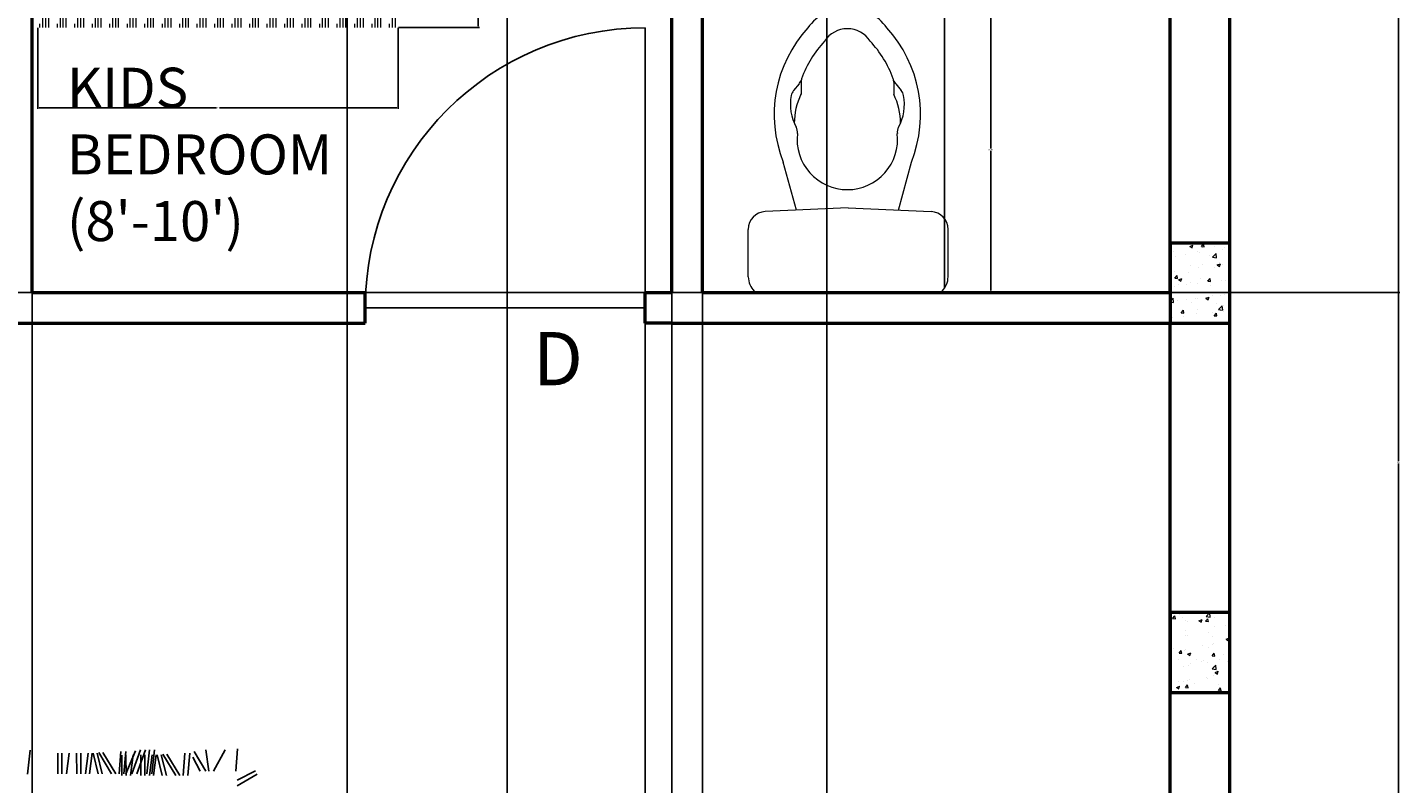
# Model space of a CAD drawing. Units: inches. Extents: x -1517 to -668, y -425 to 52.
# Tile 7 of 13: x -1186 to -980, y -176 to -63. Entities that reach past the tile are written whole.
import ezdxf

# ---------------------------------------------------------------- set-up
doc = ezdxf.new("R2010")
doc.units = ezdxf.units.IN
doc.header["$MEASUREMENT"] = 0
for name, color, linetype, lineweight in [('A-ANNO-DIMS', 2, 'Continuous', 18), ('A-ANNO-TEXT', 7, 'Continuous', 18), ('A-AREA-IDEN', 7, 'Continuous', 25), ('A-COLS-PATT', 252, 'Continuous', 13), ('A-FLOR-FIXT', 9, 'Continuous', 18), ('column', 7, 'Continuous', 50), ('doors', 25, 'Continuous', 25), ('furniture block', 8, 'Continuous', 18), ('walls', 240, 'Continuous', 50)]:
    doc.layers.add(name, color=color, linetype=linetype, lineweight=lineweight)
doc.layers.add('辅助线', color=1, linetype='Continuous')
doc.styles.get("Standard").update_dxf_attribs({"font": 'arial.ttf'})
doc.dimstyles.get("Standard").update_dxf_attribs({"dimtxt": 0.18, "dimasz": 0.18, "dimexe": 0.18, "dimexo": 0.0625, "dimgap": 0.09, "dimtad": 0, "dimtih": 1, "dimtoh": 1, "dimdec": 4, "dimzin": 0, "dimdsep": 46, "dimlunit": 4, "dimtxsty": 'Standard', "dimcen": 0.09, "dimadec": 0, "dimazin": 0, "dimtfac": 1, "dimtdec": 4, "dimtofl": 0, "dimtmove": 0, "dimatfit": 3, "dimfxl": 1, "dimtolj": 1, "dimtzin": 0, "dimarcsym": 0})

# ---------------------------------------------------------------- blocks, each defined once
blk = doc.blocks.new('door 3.6ft')
for p, q in [((0, 42), (0, 0)), ((0, 0), (42, 0))]:
    blk.add_line(p, q)
blk.add_arc((0, 0), 42, 0, 90)
blk = doc.blocks.new('column')
for p, q in [((0, 9), (0, 0)), ((12, 9), (0, 9)), ((12, 0), (12, 9)), ((0, 0), (12, 0))]:
    blk.add_line(p, q)
blk = doc.blocks.new('A$C62731D1C')
for p, q in [((0.046, 0, 0.6857), (0.046, 0.1658, 0.6857)), ((1.471, 0, 0.6857), (1.471, 0.1658, 0.6857)), ((0.021, 0, 0.6857), (0.021, 0.0658, 0.6857)), ((0.0335, 0, 0.6857), (0.0335, 0.1158, 0.6857)), ((0.096, 0, 0.6857), (0.096, 0.0658, 0.6857)), ((0.1085, 0, 0.6857), (0.1085, 0.1, 0.6857)), ((0.121, 0, 0.6857), (0.121, 0.1, 0.6857)), ((0.171, 0, 0.6857), (0.171, 0.0658, 0.6857)), ((0.1835, 0, 0.6857), (0.1835, 0.1, 0.6857)), ((0.196, 0, 0.6857), (0.196, 0.1, 0.6857)), ((0.246, 0, 0.6857), (0.246, 0.0658, 0.6857)), ((0.2585, 0, 0.6857), (0.2585, 0.1, 0.6857)), ((0.271, 0, 0.6857), (0.271, 0.1, 0.6857)), ((0.321, 0, 0.6857), (0.321, 0.0658, 0.6857)), ((0.3335, 0, 0.6857), (0.3335, 0.1, 0.6857)), ((0.346, 0, 0.6857), (0.346, 0.1, 0.6857)), ((0.396, 0, 0.6857), (0.396, 0.0658, 0.6857)), ((0.4085, 0, 0.6857), (0.4085, 0.1, 0.6857)), ((0.421, 0, 0.6857), (0.421, 0.1, 0.6857)), ((0.471, 0, 0.6857), (0.471, 0.0658, 0.6857)), ((0.4835, 0, 0.6857), (0.4835, 0.1, 0.6857)), ((0.496, 0, 0.6857), (0.496, 0.1, 0.6857)), ((0.546, 0, 0.6857), (0.546, 0.0658, 0.6857)), ((0.5585, 0, 0.6857), (0.5585, 0.1, 0.6857)), ((0.571, 0, 0.6857), (0.571, 0.1, 0.6857)), ((0.621, 0, 0.6857), (0.621, 0.0658, 0.6857)), ((0.6335, 0, 0.6857), (0.6335, 0.1, 0.6857)), ((0.646, 0, 0.6857), (0.646, 0.1, 0.6857)), ((0.696, 0, 0.6857), (0.696, 0.0658, 0.6857)), ((0.7085, 0, 0.6857), (0.7085, 0.1, 0.6857)), ((0.721, 0, 0.6857), (0.721, 0.1, 0.6857)), ((0.771, 0, 0.6857), (0.771, 0.0658, 0.6857)), ((0.7835, 0, 0.6857), (0.7835, 0.1, 0.6857)), ((0.796, 0, 0.6857), (0.796, 0.1, 0.6857)), ((0.846, 0, 0.6857), (0.846, 0.0658, 0.6857)), ((0.8585, 0, 0.6857), (0.8585, 0.1, 0.6857)), ((0.871, 0, 0.6857), (0.871, 0.1, 0.6857)), ((0.921, 0, 0.6857), (0.921, 0.0658, 0.6857)), ((0.9335, 0, 0.6857), (0.9335, 0.1, 0.6857)), ((0.946, 0, 0.6857), (0.946, 0.1, 0.6857)), ((0.996, 0, 0.6857), (0.996, 0.0658, 0.6857)), ((1.0085, 0, 0.6857), (1.0085, 0.1, 0.6857)), ((1.021, 0, 0.6857), (1.021, 0.1, 0.6857)), ((1.071, 0, 0.6857), (1.071, 0.0658, 0.6857)), ((1.0835, 0, 0.6857), (1.0835, 0.1, 0.6857)), ((1.096, 0, 0.6857), (1.096, 0.1, 0.6857)), ((1.146, 0, 0.6857), (1.146, 0.0658, 0.6857)), ((1.1585, 0, 0.6857), (1.1585, 0.1, 0.6857)), ((1.171, 0, 0.6857), (1.171, 0.1, 0.6857)), ((1.221, 0, 0.6857), (1.221, 0.0658, 0.6857)), ((1.2335, 0, 0.6857), (1.2335, 0.1, 0.6857)), ((1.246, 0, 0.6857), (1.246, 0.1, 0.6857)), ((1.296, 0, 0.6857), (1.296, 0.0658, 0.6857)), ((1.3085, 0, 0.6857), (1.3085, 0.1, 0.6857)), ((1.321, 0, 0.6857), (1.321, 0.1, 0.6857)), ((1.371, 0, 0.6857), (1.371, 0.0658, 0.6857)), ((1.3835, 0, 0.6857), (1.3835, 0.1, 0.6857)), ((1.396, 0, 0.6857), (1.396, 0.1, 0.6857)), ((1.446, 0, 0.6857), (1.446, 0.0658, 0.6857)), ((1.4585, 0, 0.6857), (1.4585, 0.1158, 0.6857)), ((1.521, 0, 0.6857), (1.521, 0.0658, 0.6857)), ((1.5335, 0, 0.6857), (1.5335, 0.1158, 0.6857)), ((0.0085, 0, 0.6857), (0.0085, 0.0158, 0.6857)), ((0.0835, 0, 0.6857), (0.0835, 0.0158, 0.6857)), ((0.1585, 0, 0.6857), (0.1585, 0.0158, 0.6857)), ((0.2335, 0, 0.6857), (0.2335, 0.0158, 0.6857)), ((0.3085, 0, 0.6857), (0.3085, 0.0158, 0.6857)), ((0.3835, 0, 0.6857), (0.3835, 0.0158, 0.6857)), ((0.4585, 0, 0.6857), (0.4585, 0.0158, 0.6857)), ((0.5335, 0, 0.6857), (0.5335, 0.0158, 0.6857)), ((0.6085, 0, 0.6857), (0.6085, 0.0158, 0.6857)), ((0.6835, 0, 0.6857), (0.6835, 0.0158, 0.6857)), ((0.7585, 0, 0.6857), (0.7585, 0.0158, 0.6857)), ((0.8335, 0, 0.6857), (0.8335, 0.0158, 0.6857)), ((0.9085, 0, 0.6857), (0.9085, 0.0158, 0.6857)), ((0.9835, 0, 0.6857), (0.9835, 0.0158, 0.6857)), ((1.0585, 0, 0.6857), (1.0585, 0.0158, 0.6857)), ((1.1335, 0, 0.6857), (1.1335, 0.0158, 0.6857)), ((1.2085, 0, 0.6857), (1.2085, 0.0158, 0.6857)), ((1.2835, 0, 0.6857), (1.2835, 0.0158, 0.6857)), ((1.3585, 0, 0.6857), (1.3585, 0.0158, 0.6857)), ((1.4335, 0, 0.6857), (1.4335, 0.0158, 0.6857)), ((1.5085, 0, 0.6857), (1.5085, 0.0158, 0.6857))]:
    blk.add_line(p, q)
blk = doc.blocks.new('A$C0E6D7E3D')
blk.add_blockref('A$C62731D1C', (0, 0))
blk = doc.blocks.new('A$C1308471B')
at = {"ltscale": 20}
for p, q in [((0.0354, 0.4793), (0.1495, 0.4793)), ((0, 0.4607), (0, 0.0186)), ((0.2013, 0.2397), (0.1923, 0.4384)), ((0.1957, 0.3639), (0.3109, 0.3953)), ((0.4982, 0.3575), (0.4822, 0.3709)), ((0.5021, 0.3528), (0.4724, 0.3528)), ((0.2013, 0.2397), (0.1923, 0.0409)), ((0.1959, 0.1193), (0.3109, 0.0879)), ((0.5021, 0.1304), (0.4724, 0.1304)), ((0.4982, 0.1257), (0.4822, 0.1123)), ((0.0354, 0), (0.1495, 0))]:
    blk.add_line(p, q, dxfattribs=at)
for centre, radius, start, end in [((0.006, 0.4607), 0.006, 136.5269, 180), ((0.0354, 0.4328), 0.0465, 90, 136.5269), ((0.1495, 0.4365), 0.0429, 2.5755, 90), ((0.4248, 0.1104), 0.3068, 47.4135, 111.7924), ((0.3823, 0.3868), 0.0255, 263.3523, 298.5742), ((0.4494, 0.2636), 0.1148, 79.3968, 118.5742), ((0.405, 0.2159), 0.153, 63.502, 90.4522), ((0.4658, 0.3513), 0.0255, 50, 79.3968), ((0.3654, 0.2416), 0.1206, 83.3523, 180), ((0.5146, 0.377), 0.0255, 230, 251.3881), ((0.5021, 0.3273), 0.0255, 70.3751, 90), ((0.4248, 0.1104), 0.2558, 46.612, 70.3751), ((0.5654, 0.2416), 0.116, 0, 54.7115), ((0.5654, 0.2416), 0.065, 0, 57.2974), ((0.3654, 0.2416), 0.1206, 180, 276.6477), ((0.5654, 0.2416), 0.065, 302.7026, 0), ((0.5654, 0.2416), 0.116, 305.2885, 0), ((0.4248, 0.3728), 0.2558, 289.6249, 313.388), ((0.4248, 0.3728), 0.3068, 248.2076, 312.5865), ((0.5021, 0.1559), 0.0255, 270, 289.6249), ((0.3823, 0.0964), 0.0255, 61.4258, 96.6477), ((0.4494, 0.2196), 0.1148, 241.4258, 280.6032), ((0.405, 0.2673), 0.153, 269.5478, 296.498), ((0.4658, 0.1319), 0.0255, 280.6032, 310), ((0.5146, 0.1062), 0.0255, 108.6119, 130), ((0.1495, 0.0429), 0.0429, 270, 357.4245), ((0.006, 0.0186), 0.006, 180, 223.4731), ((0.0354, 0.0465), 0.0465, 223.4731, 270)]:
    blk.add_arc(centre, radius, start, end, dxfattribs=at)
blk = doc.blocks.new('A$C2A9E403C')
at = {"layer": '辅助线'}
for p, q in [((-1.0661, 2.2523), (-1.0302, 2.1808)), ((-1.0533, 2.2588), (-1.0079, 2.1808)), ((-1.1526, 2.1822), (-1.0649, 2.175)), ((-1.1494, 2.1339), (-1.0648, 2.0871)), ((-1.1493, 2.0567), (-1.0648, 2.0692)), ((-1.1428, 2.0116), (-1.0648, 2.0569)), ((-1.1205, 2.0067), (-1.0648, 2.0347)), ((-1.1354, 1.9942), (-1.0477, 1.987)), ((-1.1354, 1.9749), (-1.0477, 1.9677)), ((-1.1321, 1.9041), (-1.0476, 1.9549)), ((-1.132, 1.888), (-1.0476, 1.9389)), ((-1.1288, 1.8816), (-1.0476, 1.902)), ((-1.1487, 1.855), (-1.0545, 1.8446)), ((-1.1288, 1.8655), (-1.0476, 1.8859)), ((-1.1288, 1.8623), (-1.0475, 1.8515)), ((-1.1288, 1.8462), (-1.0475, 1.8354)), ((-1.1486, 1.8356), (-1.0545, 1.8253)), ((-1.1486, 1.8196), (-1.0544, 1.7859)), ((-1.1486, 1.8002), (-1.0544, 1.7666)), ((-1.1287, 1.8172), (-1.0475, 1.8173)), ((-1.1287, 1.8011), (-1.0475, 1.8012)), ((-1.1454, 1.7809), (-1.0544, 1.7424)), ((-1.1421, 1.7423), (-1.0544, 1.7351)), ((-1.1287, 1.7721), (-1.0474, 1.7614)), ((-1.1287, 1.7432), (-1.0474, 1.7433)), ((-1.1421, 1.723), (-1.0544, 1.7158)), ((-1.1388, 1.6522), (-1.0544, 1.703)), ((-1.1388, 1.6361), (-1.0543, 1.6869)), ((-1.1286, 1.7271), (-1.0474, 1.7272)), ((-1.1355, 1.6296), (-1.0543, 1.6501)), ((-1.1355, 1.6135), (-1.0543, 1.634)), ((-1.1355, 1.6103), (-1.0542, 1.5996)), ((-1.1355, 1.5942), (-1.0542, 1.5835)), ((-1.1355, 1.5653), (-1.0542, 1.5654)), ((-1.1354, 1.5492), (-1.0542, 1.5493)), ((-1.1354, 1.5202), (-1.0541, 1.5094)), ((-1.1354, 1.4912), (-1.0541, 1.4913)), ((-1.1354, 1.4751), (-1.0541, 1.4752)), ((-1.1481, 1.3657), (-1.0539, 1.3553))]:
    blk.add_line(p, q, dxfattribs=at)
blk = doc.blocks.new('*D30')
at = {"layer": 'A-ANNO-DIMS', "color": 0, "lineweight": -2, "transparency": 16777216}
for p, q in [((-1047.75, -59.62), (-1041.24, -59.62)), ((-1041.42, -59.8), (-1041.42, -80.76)), ((-1041.42, -102.09), (-1041.42, -81.13)), ((-1047.75, -102.27), (-1041.24, -102.27))]:
    blk.add_line(p, q, dxfattribs=at)
at = {"layer": 'A-ANNO-DIMS', "color": 0, "transparency": 16777216}
for points in [[(-1041.45, -59.8), (-1041.39, -59.8), (-1041.42, -59.62)], [(-1041.45, -102.09), (-1041.39, -102.09), (-1041.42, -102.27)]]:
    blk.add_solid(points, dxfattribs=at)
at = {"layer": 'Defpoints', "color": 0, "transparency": 16777216}
for p in [(-1047.82, -59.62), (-1041.42, -59.62), (-1047.82, -102.27)]:
    blk.add_point(p, dxfattribs=at)
at = {"layer": 'A-ANNO-DIMS', "color": 0, "transparency": 16777216, "insert": (-1041.42, -80.94), "char_height": 0.18, "attachment_point": 5}
blk.add_mtext('\\A1;WC 43', dxfattribs=at)
blk = doc.blocks.new('*D36')
at = {"layer": 'A-ANNO-DIMS', "color": 0, "lineweight": -2, "transparency": 16777216}
for p, q in [((-1130.31, 17.63), (-1118.16, 17.63)), ((-1118.34, 17.45), (-1118.34, -22.31)), ((-1118.34, -62.44), (-1118.34, -22.68)), ((-1130.31, -62.62), (-1118.16, -62.62))]:
    blk.add_line(p, q, dxfattribs=at)
at = {"layer": 'A-ANNO-DIMS', "color": 0, "transparency": 16777216}
for points in [[(-1118.37, 17.45), (-1118.31, 17.45), (-1118.34, 17.63)], [(-1118.37, -62.44), (-1118.31, -62.44), (-1118.34, -62.62)]]:
    blk.add_solid(points, dxfattribs=at)
at = {"layer": 'Defpoints', "color": 0, "transparency": 16777216}
for p in [(-1130.37, 17.63), (-1118.34, 17.63), (-1130.37, -62.62)]:
    blk.add_point(p, dxfattribs=at)
at = {"layer": 'A-ANNO-DIMS', "color": 0, "transparency": 16777216, "insert": (-1118.34, -22.5), "char_height": 0.18, "attachment_point": 5}
blk.add_mtext("\\A1;CHILD'S BED 80", dxfattribs=at)
blk = doc.blocks.new('*D37')
at = {"layer": 'A-ANNO-DIMS', "color": 0, "lineweight": -2, "transparency": 16777216}
for p, q in [((-1184.44, -62.69), (-1184.44, -74.84)), ((-1130.37, -62.69), (-1130.37, -74.84)), ((-1184.26, -74.66), (-1157.62, -74.66)), ((-1130.55, -74.66), (-1157.19, -74.66))]:
    blk.add_line(p, q, dxfattribs=at)
at = {"layer": 'A-ANNO-DIMS', "color": 0, "transparency": 16777216}
for points in [[(-1184.26, -74.63), (-1184.26, -74.69), (-1184.44, -74.66)], [(-1130.55, -74.63), (-1130.55, -74.69), (-1130.37, -74.66)]]:
    blk.add_solid(points, dxfattribs=at)
at = {"layer": 'Defpoints', "color": 0, "transparency": 16777216}
for p in [(-1184.44, -62.62), (-1130.37, -62.62), (-1130.37, -74.66)]:
    blk.add_point(p, dxfattribs=at)
at = {"layer": 'A-ANNO-DIMS', "color": 0, "transparency": 16777216, "insert": (-1157.41, -74.66), "char_height": 0.18, "attachment_point": 5}
blk.add_mtext('\\A1;54', dxfattribs=at)
blk = doc.blocks.new('*D46')
at = {"layer": 'A-ANNO-DIMS', "color": 0, "lineweight": -2, "transparency": 16777216}
for p, q in [((-1005.44, 26.63), (-980.02, 26.63)), ((-980.2, 26.45), (-980.2, -127.69)), ((-980.2, -282.19), (-980.2, -128.05)), ((-1005.44, -282.37), (-980.02, -282.37))]:
    blk.add_line(p, q, dxfattribs=at)
at = {"layer": 'A-ANNO-DIMS', "color": 0, "transparency": 16777216}
for points in [[(-980.23, 26.45), (-980.17, 26.45), (-980.2, 26.63)], [(-980.23, -282.19), (-980.17, -282.19), (-980.2, -282.37)]]:
    blk.add_solid(points, dxfattribs=at)
at = {"layer": 'Defpoints', "color": 0, "transparency": 16777216}
for p in [(-1005.5, 26.63), (-1005.5, -282.37), (-980.2, -282.37)]:
    blk.add_point(p, dxfattribs=at)
at = {"layer": 'A-ANNO-DIMS', "color": 0, "transparency": 16777216, "insert": (-980.2, -127.87), "char_height": 0.18, "attachment_point": 5}
blk.add_mtext('\\A1;309', dxfattribs=at)
blk = doc.blocks.new('*D49')
at = {"layer": 'A-ANNO-DIMS', "color": 0, "lineweight": -2, "transparency": 16777216}
for p, q in [((-1185.3, -102.43), (-1185.3, -376.85)), ((-1089.3, -102.43), (-1089.3, -376.85)), ((-1185.12, -376.67), (-1137.52, -376.67)), ((-1089.48, -376.67), (-1137.08, -376.67))]:
    blk.add_line(p, q, dxfattribs=at)
at = {"layer": 'A-ANNO-DIMS', "color": 0, "transparency": 16777216}
for points in [[(-1185.12, -376.64), (-1185.12, -376.7), (-1185.3, -376.67)], [(-1089.48, -376.64), (-1089.48, -376.7), (-1089.3, -376.67)]]:
    blk.add_solid(points, dxfattribs=at)
at = {"layer": 'Defpoints', "color": 0, "transparency": 16777216}
for p in [(-1185.3, -102.37), (-1089.3, -102.37), (-1089.3, -376.67)]:
    blk.add_point(p, dxfattribs=at)
at = {"layer": 'A-ANNO-DIMS', "color": 0, "transparency": 16777216, "insert": (-1137.3, -376.67), "char_height": 0.18, "attachment_point": 5}
blk.add_mtext('\\A1;96', dxfattribs=at)
blk = doc.blocks.new('*D50')
at = {"layer": 'A-ANNO-DIMS', "color": 0, "lineweight": -2, "transparency": 16777216}
for p, q in [((-1084.7, -102.43), (-1084.7, -376.85)), ((-1014.5, -102.43), (-1014.5, -376.85)), ((-1084.52, -376.67), (-1049.93, -376.67)), ((-1014.68, -376.67), (-1049.28, -376.67))]:
    blk.add_line(p, q, dxfattribs=at)
at = {"layer": 'A-ANNO-DIMS', "color": 0, "transparency": 16777216}
for points in [[(-1084.52, -376.64), (-1084.52, -376.7), (-1084.7, -376.67)], [(-1014.68, -376.64), (-1014.68, -376.7), (-1014.5, -376.67)]]:
    blk.add_solid(points, dxfattribs=at)
at = {"layer": 'Defpoints', "color": 0, "transparency": 16777216}
for p in [(-1084.7, -102.37), (-1014.5, -102.37), (-1014.5, -376.67)]:
    blk.add_point(p, dxfattribs=at)
at = {"layer": 'A-ANNO-DIMS', "color": 0, "transparency": 16777216, "insert": (-1049.6, -376.67), "char_height": 0.18, "attachment_point": 5}
blk.add_mtext('\\A1;70.2', dxfattribs=at)
blk = doc.blocks.new('*D53')
at = {"layer": 'A-ANNO-DIMS', "color": 0, "lineweight": -2, "transparency": 16777216}
for p, q in [((-1242.5, -153.31), (-1242.5, 52.11)), ((-1242.32, 51.93), (-1128.79, 51.93)), ((-1014.68, 51.93), (-1128.21, 51.93)), ((-1014.5, -150.31), (-1014.5, 52.11))]:
    blk.add_line(p, q, dxfattribs=at)
at = {"layer": 'A-ANNO-DIMS', "color": 0, "transparency": 16777216}
for points in [[(-1242.32, 51.96), (-1242.32, 51.9), (-1242.5, 51.93)], [(-1014.68, 51.96), (-1014.68, 51.9), (-1014.5, 51.93)]]:
    blk.add_solid(points, dxfattribs=at)
at = {"layer": 'Defpoints', "color": 0, "transparency": 16777216}
for p in [(-1014.5, 51.93), (-1014.5, -150.37), (-1242.5, -153.37)]:
    blk.add_point(p, dxfattribs=at)
at = {"layer": 'A-ANNO-DIMS', "color": 0, "transparency": 16777216, "insert": (-1128.5, 51.93), "char_height": 0.18, "attachment_point": 5}
blk.add_mtext('\\A1;228', dxfattribs=at)
blk = doc.blocks.new('*D57')
at = {"layer": 'A-ANNO-DIMS', "color": 0, "lineweight": -2, "transparency": 16777216}
for p, q in [((-1114.02, -282.31), (-1114.02, 52.11)), ((-1113.84, 51.93), (-1090.24, 51.93)), ((-1066.2, 51.93), (-1089.8, 51.93)), ((-1066.02, -282.31), (-1066.02, 52.11))]:
    blk.add_line(p, q, dxfattribs=at)
at = {"layer": 'A-ANNO-DIMS', "color": 0, "transparency": 16777216}
for points in [[(-1113.84, 51.96), (-1113.84, 51.9), (-1114.02, 51.93)], [(-1066.2, 51.96), (-1066.2, 51.9), (-1066.02, 51.93)]]:
    blk.add_solid(points, dxfattribs=at)
at = {"layer": 'Defpoints', "color": 0, "transparency": 16777216}
for p in [(-1066.02, 51.93), (-1114.02, -282.37), (-1066.02, -282.37)]:
    blk.add_point(p, dxfattribs=at)
at = {"layer": 'A-ANNO-DIMS', "color": 0, "transparency": 16777216, "insert": (-1090.02, 51.93), "char_height": 0.18, "attachment_point": 5}
blk.add_mtext('\\A1;48', dxfattribs=at)
blk = doc.blocks.new('*D58')
at = {"layer": 'A-ANNO-DIMS', "color": 0, "lineweight": -2, "transparency": 16777216}
for p, q in [((-1066.02, -282.31), (-1066.02, 52.11)), ((-1065.84, 51.93), (-1036.14, 51.93)), ((-1005.68, 51.93), (-1035.38, 51.93)), ((-1005.5, -282.31), (-1005.5, 52.11))]:
    blk.add_line(p, q, dxfattribs=at)
at = {"layer": 'A-ANNO-DIMS', "color": 0, "transparency": 16777216}
for points in [[(-1065.84, 51.96), (-1065.84, 51.9), (-1066.02, 51.93)], [(-1005.68, 51.96), (-1005.68, 51.9), (-1005.5, 51.93)]]:
    blk.add_solid(points, dxfattribs=at)
at = {"layer": 'Defpoints', "color": 0, "transparency": 16777216}
for p in [(-1005.5, 51.93), (-1066.02, -282.37), (-1005.5, -282.37)]:
    blk.add_point(p, dxfattribs=at)
at = {"layer": 'A-ANNO-DIMS', "color": 0, "transparency": 16777216, "insert": (-1035.76, 51.93), "char_height": 0.18, "attachment_point": 5}
blk.add_mtext('\\A1;60.51', dxfattribs=at)
blk = doc.blocks.new('*D65')
at = {"layer": 'A-ANNO-DIMS', "color": 0, "lineweight": -2, "transparency": 16777216}
for p, q in [((-1138.02, -282.31), (-1138.02, 52.11)), ((-1137.84, 51.93), (-1126.24, 51.93)), ((-1114.2, 51.93), (-1125.8, 51.93)), ((-1114.02, -282.31), (-1114.02, 52.11))]:
    blk.add_line(p, q, dxfattribs=at)
at = {"layer": 'A-ANNO-DIMS', "color": 0, "transparency": 16777216}
for points in [[(-1137.84, 51.96), (-1137.84, 51.9), (-1138.02, 51.93)], [(-1114.2, 51.96), (-1114.2, 51.9), (-1114.02, 51.93)]]:
    blk.add_solid(points, dxfattribs=at)
at = {"layer": 'Defpoints', "color": 0, "transparency": 16777216}
for p in [(-1114.02, 51.93), (-1138.02, -282.37), (-1114.02, -282.37)]:
    blk.add_point(p, dxfattribs=at)
at = {"layer": 'A-ANNO-DIMS', "color": 0, "transparency": 16777216, "insert": (-1126.02, 51.93), "char_height": 0.18, "attachment_point": 5}
blk.add_mtext('\\A1;24', dxfattribs=at)
blk = doc.blocks.new('*D70')
at = {"layer": 'A-ANNO-DIMS', "color": 0, "lineweight": -2, "transparency": 16777216}
for p, q in [((-1089.3, -102.43), (-1089.3, -376.85)), ((-1093.3, -107.03), (-1093.3, -376.85)), ((-1093.12, -376.67), (-1091.46, -376.67)), ((-1089.48, -376.67), (-1091.15, -376.67))]:
    blk.add_line(p, q, dxfattribs=at)
at = {"layer": 'A-ANNO-DIMS', "color": 0, "transparency": 16777216}
for points in [[(-1093.12, -376.64), (-1093.12, -376.7), (-1093.3, -376.67)], [(-1089.48, -376.64), (-1089.48, -376.7), (-1089.3, -376.67)]]:
    blk.add_solid(points, dxfattribs=at)
at = {"layer": 'Defpoints', "color": 0, "transparency": 16777216}
for p in [(-1089.3, -102.37), (-1093.3, -106.97), (-1089.3, -376.67)]:
    blk.add_point(p, dxfattribs=at)
at = {"layer": 'A-ANNO-DIMS', "color": 0, "transparency": 16777216, "insert": (-1091.3, -376.67), "char_height": 0.18, "attachment_point": 5}
blk.add_mtext('\\A1;4', dxfattribs=at)
blk = doc.blocks.new('*D72')
at = {"layer": 'A-ANNO-DIMS', "color": 0, "lineweight": -2, "transparency": 16777216}
for p, q in [((-1285.84, -16.28), (-980.02, -16.28)), ((-980.2, -16.46), (-980.2, -59.14)), ((-980.2, -102.19), (-980.2, -59.51)), ((-1285.84, -102.37), (-980.02, -102.37))]:
    blk.add_line(p, q, dxfattribs=at)
at = {"layer": 'A-ANNO-DIMS', "color": 0, "transparency": 16777216}
for points in [[(-980.23, -16.46), (-980.17, -16.46), (-980.2, -16.28)], [(-980.23, -102.19), (-980.17, -102.19), (-980.2, -102.37)]]:
    blk.add_solid(points, dxfattribs=at)
at = {"layer": 'Defpoints', "color": 0, "transparency": 16777216}
for p in [(-1285.9, -16.28), (-1285.9, -102.37), (-980.2, -102.37)]:
    blk.add_point(p, dxfattribs=at)
at = {"layer": 'A-ANNO-DIMS', "color": 0, "transparency": 16777216, "insert": (-980.2, -59.33), "char_height": 0.18, "attachment_point": 5}
blk.add_mtext('\\A1;86.09', dxfattribs=at)
blk = doc.blocks.new('*D73')
at = {"layer": 'A-ANNO-DIMS', "color": 0, "lineweight": -2, "transparency": 16777216}
for p, q in [((-1089.37, -16.37), (-1516.98, -16.37)), ((-1516.8, -16.55), (-1516.8, -59.19)), ((-1516.8, -102.19), (-1516.8, -59.55)), ((-1089.37, -102.37), (-1516.98, -102.37))]:
    blk.add_line(p, q, dxfattribs=at)
at = {"layer": 'A-ANNO-DIMS', "color": 0, "transparency": 16777216}
for points in [[(-1516.83, -16.55), (-1516.77, -16.55), (-1516.8, -16.37)], [(-1516.83, -102.19), (-1516.77, -102.19), (-1516.8, -102.37)]]:
    blk.add_solid(points, dxfattribs=at)
at = {"layer": 'Defpoints', "color": 0, "transparency": 16777216}
for p in [(-1089.3, -16.37), (-1516.8, -102.37), (-1089.3, -102.37)]:
    blk.add_point(p, dxfattribs=at)
at = {"layer": 'A-ANNO-DIMS', "color": 0, "transparency": 16777216, "insert": (-1516.8, -59.37), "char_height": 0.18, "attachment_point": 5}
blk.add_mtext('\\A1;86', dxfattribs=at)
blk = doc.blocks.new('*D78')
at = {"layer": 'A-ANNO-DIMS', "color": 0, "lineweight": -2, "transparency": 16777216}
for p, q in [((-1048.34, -101.65), (-1048.34, 52.11)), ((-1048.16, 51.93), (-1031.89, 51.93)), ((-1014.68, 51.93), (-1030.96, 51.93)), ((-1014.5, -102.31), (-1014.5, 52.11))]:
    blk.add_line(p, q, dxfattribs=at)
at = {"layer": 'A-ANNO-DIMS', "color": 0, "transparency": 16777216}
for points in [[(-1048.16, 51.96), (-1048.16, 51.9), (-1048.34, 51.93)], [(-1014.68, 51.96), (-1014.68, 51.9), (-1014.5, 51.93)]]:
    blk.add_solid(points, dxfattribs=at)
at = {"layer": 'Defpoints', "color": 0, "transparency": 16777216}
for p in [(-1048.34, 51.93), (-1048.34, -101.71), (-1014.5, -102.37)]:
    blk.add_point(p, dxfattribs=at)
at = {"layer": 'A-ANNO-DIMS', "color": 0, "transparency": 16777216, "insert": (-1031.42, 51.93), "char_height": 0.18, "attachment_point": 5}
blk.add_mtext('\\A1;33.835', dxfattribs=at)

msp = doc.modelspace()

# ---------------------------------------------------------------- hatches: boundary and pattern name
at = {"layer": 'A-COLS-PATT'}
h = msp.add_hatch(dxfattribs=at)
h.set_pattern_fill('AR-CONC', color=256, scale=0.69)
h.set_pattern_definition([(50, (0, 0), (4.949095, -0.43299), [0.5175, -5.6925]), (355, (0, 0), (-0.957384, 5.190126), [0.414, -4.554]), (100.45144, (0.4124, -0.036), (3.99171, 4.757136), [0.439807, -4.83788]), (46.1842, (0, 1.38), (7.363965, -1.142083), [0.77625, -8.53875]), (96.6356, (0.614, 1.285), (6.449167, 6.72142), [0.65971, -7.256825]), (351.1842, (0, 1.38), (6.44917, 6.72142), [0.621, -6.831]), (21, (0.69, 1.035), (4.118659, -2.77807), [0.5175, -5.6925]), (326, (0.69, 1.035), (1.678876, 5.003535), [0.414, -4.554]), (71.45144, (1.033, 0.8035), (5.797534, 2.225465), [0.439807, -4.83788]), (37.5, (0, 0), (0.083903, 2.2969676), [0, -4.4988, 0, -4.623, 0, -4.57125]), (7.5, (0, 0), (1.81518, 2.721441), [0, -2.6358, 0, -4.3953, 0, -1.74225]), (327.5, (-1.5387, 0), (3.6833748, -0.1556286), [0, -1.725, 0, -5.382, 0, -7.1415]), (317.5, (-2.2287, 0), (4.023985, 0.690724), [0, -2.2425, 0, -3.5742, 0, -5.0715])])
h.paths.add_polyline_path([(-1005.5037, -94.97), (-1014.5037, -94.97), (-1014.5037, -106.97), (-1005.5037, -106.97)])
h.paths.add_polyline_path([(-1005.5037, -150.37), (-1014.5037, -150.37), (-1014.5037, -162.37), (-1005.5037, -162.37)])

# ---------------------------------------------------------------- linework, layer by layer
at = {"layer": 'walls'}
for p, q in [((-1005.5037, -282.37), (-1005.5037, 26.63)), ((-1185.3037, -102.37), (-1185.3037, 17.63)), ((-1014.5037, -102.37), (-1014.5037, 17.63)), ((-1089.3037, -102.37), (-1089.3037, -16.37)), ((-1084.7037, -102.37), (-1084.7037, -16.2817)), ((-1185.3037, -102.37), (-1135.3037, -102.37)), ((-1135.3037, -106.97), (-1135.3037, -102.37)), ((-1093.3037, -106.97), (-1093.3037, -102.37)), ((-1093.3037, -102.37), (-1089.3037, -102.37)), ((-1084.7037, -102.37), (-1014.5037, -102.37)), ((-1285.9037, -106.97), (-1185.3037, -106.97)), ((-1185.3037, -106.97), (-1135.3037, -106.97)), ((-1089.3037, -106.97), (-1093.3037, -106.97)), ((-1089.3037, -106.97), (-1084.7037, -106.97)), ((-1084.7037, -106.97), (-1014.5037, -106.97)), ((-1014.5037, -273.37), (-1014.5037, -106.97))]:
    msp.add_line(p, q, dxfattribs=at)

# ---------------------------------------------------------------- block references
at = {"layer": 'A-FLOR-FIXT', "xscale": 62.5850366996167, "yscale": 62.5850366996167, "zscale": 62.5850366996167, "rotation": 89.99999999999999}
msp.add_blockref('A$C1308471B', (-1047.8167, -102.2668), dxfattribs=at)
at = {"layer": 'column', "rotation": 270}
for p in [(-1014.5037, -94.97), (-1014.5037, -150.37)]:
    msp.add_blockref('column', p, dxfattribs=at)
at = {"layer": 'doors', "xscale": -1}
msp.add_blockref('door 3.6ft', (-1093.3037, -104.67), dxfattribs=at)
at = {"layer": 'furniture block', "xscale": 34.99562554665724, "yscale": 34.99562554665724, "zscale": 34.99562554665724}
msp.add_blockref('A$C0E6D7E3D', (-1184.4382, -62.6234), dxfattribs=at)
at = {"layer": 'furniture block', "xscale": 38.16622643712981, "yscale": 38.16622643712981, "zscale": 38.16622643712981, "rotation": 270}
msp.add_blockref('A$C2A9E403C', (-1237.7606, -214.8323), dxfattribs=at)

# ---------------------------------------------------------------- texts
at = {"layer": 'A-ANNO-TEXT', "insert": (-1110.1427, -108.3056), "char_height": 8, "attachment_point": 1}
msp.add_mtext_dynamic_manual_height_columns('{\\fArial|b1|i0|c0|p34;D}', width=23.131632, gutter_width=1, heights=[0], dxfattribs=at)
at = {"layer": 'A-AREA-IDEN', "insert": (-1180.0847, -68.6599), "char_height": 6, "attachment_point": 1}
msp.add_mtext_dynamic_manual_height_columns("{\\fArial|b1|i0|c0|p34;KIDS BEDROOM\\P(8'-10')}", width=47.827229, gutter_width=1, heights=[0], dxfattribs=at)

# ---------------------------------------------------------------- dimensions: what is measured, and where the dimension line sits
at = {"layer": 'A-ANNO-DIMS'}
for base, p1, p2, override, picture, middle in [((-1014.5037, 51.93), (-1242.5037, -153.37), (-1014.5037, -150.37), {"dimdec": 0, "dimlfac": 1, "dimrnd": 0, "dimzin": 0, "dimdsep": 46, "dimlunit": 2}, '*D53', (-1128.5037, 51.93)), ((-1114.0183, 51.93), (-1138.0183, -282.37), (-1114.0183, -282.37), {"dimdec": 0, "dimlfac": 1, "dimrnd": 0, "dimzin": 0, "dimdsep": 46, "dimlunit": 2}, '*D65', (-1126.0183, 51.93)), ((-1066.0183, 51.93), (-1114.0183, -282.37), (-1066.0183, -282.37), {"dimdec": 0, "dimlfac": 1, "dimrnd": 0, "dimzin": 0, "dimdsep": 46, "dimlunit": 2}, '*D57', (-1090.0183, 51.93)), ((-1005.5037, 51.93), (-1066.0183, -282.37), (-1005.5037, -282.37), {"dimdec": 2, "dimlfac": 1, "dimrnd": 0, "dimzin": 0, "dimdsep": 46, "dimlunit": 2}, '*D58', (-1035.761, 51.93)), ((-1048.3383, 51.93), (-1014.5037, -102.37), (-1048.3383, -101.7142), {"dimdec": 3, "dimlfac": 1, "dimrnd": 0, "dimzin": 0, "dimdsep": 46, "dimlunit": 2}, '*D78', (-1031.421, 51.93)), ((-1130.374, -74.6614), (-1184.4382, -62.6234), (-1130.374, -62.6234), {"dimdec": 0, "dimlfac": 1, "dimrnd": 0, "dimzin": 0, "dimdsep": 46, "dimlunit": 2}, '*D37', (-1157.4061, -74.6614)), ((-1089.3037, -376.67), (-1185.3037, -102.37), (-1089.3037, -102.37), {"dimdec": 0, "dimlfac": 1, "dimrnd": 0, "dimzin": 0, "dimdsep": 46, "dimlunit": 2}, '*D49', (-1137.3037, -376.67)), ((-1089.3037, -376.67), (-1093.3037, -106.97), (-1089.3037, -102.37), {"dimdec": 0, "dimlfac": 1, "dimrnd": 0, "dimzin": 0, "dimdsep": 46, "dimlunit": 2}, '*D70', (-1091.3037, -376.67)), ((-1014.5037, -376.67), (-1084.7037, -102.37), (-1014.5037, -102.37), {"dimdec": 1, "dimlfac": 1, "dimrnd": 0, "dimzin": 0, "dimdsep": 46, "dimlunit": 2}, '*D50', (-1049.6037, -376.67))]:
    dim = msp.add_linear_dim(base=base, p1=p1, p2=p2, dimstyle='Standard', override=override, dxfattribs=at)
    dim.commit()
    dim.dimension.update_dxf_attribs({"geometry": picture, "text_midpoint": middle})
for base, p1, p2, override, picture, middle in [((-980.2037, -282.37), (-1005.5037, 26.63), (-1005.5037, -282.37), {"dimdec": 0, "dimlfac": 1, "dimrnd": 0, "dimzin": 0, "dimdsep": 46, "dimlunit": 2}, '*D46', (-980.2037, -127.87)), ((-1516.8037, -102.37), (-1089.3037, -16.37), (-1089.3037, -102.37), {"dimdec": 0, "dimlfac": 1, "dimrnd": 0, "dimzin": 0, "dimdsep": 46, "dimlunit": 2}, '*D73', (-1516.8037, -59.37)), ((-980.2037, -102.37), (-1285.9037, -16.2817), (-1285.9037, -102.37), {"dimdec": 2, "dimlfac": 1, "dimrnd": 0, "dimzin": 0, "dimdsep": 46, "dimlunit": 2}, '*D72', (-980.2037, -59.3258))]:
    dim = msp.add_linear_dim(base=base, p1=p1, p2=p2, angle=90, dimstyle='Standard', override=override, dxfattribs=at)
    dim.commit()
    dim.dimension.update_dxf_attribs({"geometry": picture, "text_midpoint": middle})
for base, p1, p2, text, picture, middle in [((-1118.336, 17.63), (-1130.374, -62.6234), (-1130.374, 17.63), "CHILD'S BED <>", '*D36', (-1118.336, -22.4967)), ((-1041.4201, -59.6228), (-1047.8167, -102.2668), (-1047.8167, -59.6228), 'WC <>', '*D30', (-1041.4201, -80.9448))]:
    dim = msp.add_linear_dim(base=base, p1=p1, p2=p2, angle=90, text=text, dimstyle='Standard', override={"dimdec": 0, "dimlfac": 1, "dimrnd": 0, "dimzin": 0, "dimdsep": 46, "dimlunit": 2}, dxfattribs=at)
    dim.commit()
    dim.dimension.update_dxf_attribs({"geometry": picture, "text_midpoint": middle})

doc.saveas('drawing.dxf')
